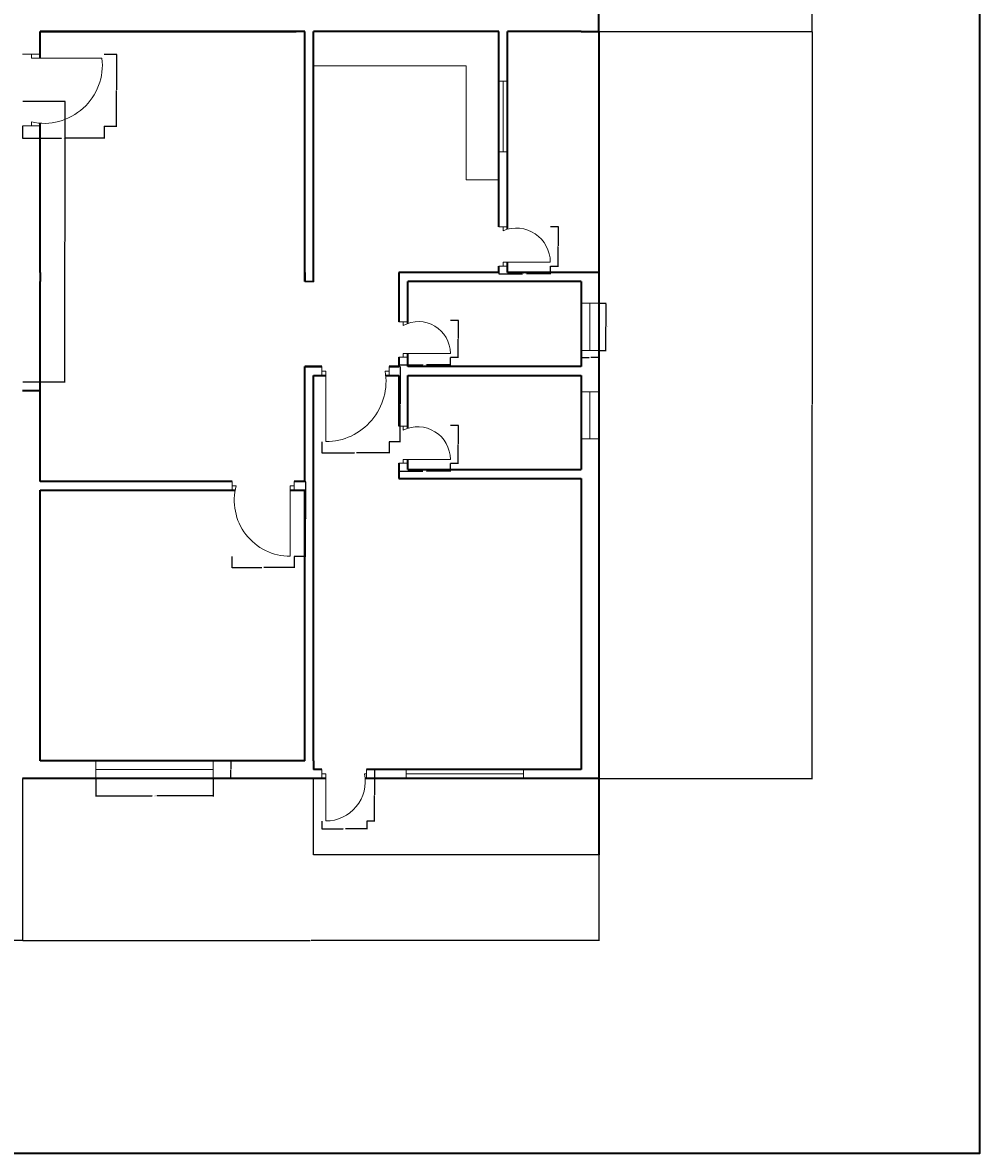
# Model space of a CAD drawing. Units: inches. Extents: x 2120 to 4013, y 1390 to 3019.
# Tile 51 of 59: x 3525 to 4013, y 1390 to 1967. Entities that reach past the tile are written whole.
import ezdxf

# ---------------------------------------------------------------- set-up
doc = ezdxf.new("R2010")
doc.units = ezdxf.units.IN
for name, color, linetype, lineweight in [('A-ANNO-DIMS', 2, 'Continuous', 18), ('A-ANNO-TTLB', 7, 'Continuous', 35), ('A-DOOR', 3, 'Continuous', 18), ('A-FLOR-CASE', 8, 'Continuous', 18), ('A-FLOR-DECK', 7, 'Continuous', 25), ('A-FURN', 8, 'Continuous', 13), ('A-GLAZ', 4, 'Continuous', 18), ('A-WALL', 7, 'Continuous', 35)]:
    doc.layers.add(name, color=color, linetype=linetype, lineweight=lineweight)
doc.styles.get("Standard").update_dxf_attribs({"font": 'arial.ttf'})
doc.dimstyles.get("Standard").update_dxf_attribs({"dimtxt": 0.18, "dimasz": 0.18, "dimexe": 0.18, "dimexo": 0.0625, "dimgap": 0.09, "dimtad": 0, "dimtih": 1, "dimtoh": 1, "dimdec": 4, "dimzin": 0, "dimdsep": 46, "dimtxsty": 'Standard', "dimcen": 0.09, "dimadec": 0, "dimazin": 0, "dimtfac": 1, "dimtdec": 4, "dimtofl": 0, "dimtmove": 0, "dimatfit": 3, "dimfxl": 1, "dimtolj": 1, "dimtzin": 0, "dimarcsym": 0})

# ---------------------------------------------------------------- blocks, each defined once
blk = doc.blocks.new('DOOR-SWING-24IN-116p21DEG')
for p, q in [((0, 18.94), (4.5, 18.94)), ((4.5, 18.94), (2.25, 18.94)), ((2.25, 18.94), (2.25, 16.94)), ((4.5, 0), (0, 0)), ((0, 0), (2.25, 0)), ((2.25, 0), (2.25, 2)), ((2.25, 2), (26.25, 2))]:
    blk.add_line(p, q)
blk.add_arc((9.6, 2), 16.65, 0, 116.20868)
blk = doc.blocks.new('DOOR-SWING-24IN-119p01DEG')
for p, q in [((0, 18.13), (4.5, 18.13)), ((4.5, 18.13), (2.25, 18.13)), ((2.25, 18.13), (2.25, 16.13)), ((0, 0), (4.5, 0)), ((2.25, 0), (2.25, 2)), ((2.25, 2), (26.25, 2)), ((4.5, 0), (2.25, 0))]:
    blk.add_line(p, q)
blk.add_arc((10.09, 2), 16.16, 0, 119.01366)
blk = doc.blocks.new('DOOR-SWING-24IN-100p95DEG')
for p, q in [((0, 26.25), (0, 21.75)), ((0, 21.75), (0, 24)), ((0, 24), (2, 24)), ((2, 24), (2, 0)), ((22.8, 24), (21.8, 24)), ((22.8, 26.25), (22.8, 21.75)), ((22.8, 21.75), (22.8, 24))]:
    blk.add_line(p, q)
blk.add_arc((2, 20.17), 20.17, 270, 10.95076)
blk = doc.blocks.new('DOOR-SWING-24IN-112p55DEG')
for p, q in [((0, 20.02), (4.5, 20.02)), ((4.5, 20.02), (2.25, 20.02)), ((2.25, 20.02), (2.25, 18.02)), ((0, 0), (4.5, 0)), ((2.25, 0), (2.25, 2)), ((2.25, 2), (26.25, 2)), ((4.5, 0), (2.25, 0))]:
    blk.add_line(p, q)
blk.add_arc((8.9, 2), 17.35, 0, 112.55014)
blk = doc.blocks.new('DOOR-SWING-36IN-99p84DEG')
for p, q in [((0, 38.25), (0, 33.75)), ((0, 33.75), (0, 38.25)), ((0, 38.25), (0, 36)), ((0, 36), (2, 36)), ((2, 36), (2, 0)), ((34.3, 36), (32.3, 36)), ((34.3, 38.25), (34.3, 33.75)), ((34.3, 33.75), (34.3, 36))]:
    blk.add_line(p, q)
blk.add_arc((2, 30.75), 30.75, 270, 9.83553)
blk = doc.blocks.new('DOOR-SWING-36IN-105p06DEG')
for p, q in [((0, 33.75), (0, 38.25)), ((0, 38.25), (0, 36)), ((0, 36), (2, 36)), ((31.6, 36), (29.6, 36)), ((29.6, 36), (29.6, 0)), ((31.6, 38.25), (31.6, 33.75)), ((31.6, 33.75), (31.6, 36))]:
    blk.add_line(p, q)
blk.add_arc((29.6, 28.58), 28.58, 164.94449, 270)
blk = doc.blocks.new('DOOR-SWING-36IN-109p07DEG')
for p, q in [((9, 36.56), (0, 36.56)), ((0, 36.56), (4.5, 36.56)), ((4.5, 36.56), (4.5, 34.56)), ((9, 36.56), (9, 36.56)), ((4.5, 34.56), (40.5, 34.56)), ((9, 0), (0, 0)), ((0, 0), (4.5, 0)), ((4.5, 0), (4.5, 2))]:
    blk.add_line(p, q)
blk.add_arc((10.9, 31.1), 29.8, 257.59275, 6.66524)
blk = doc.blocks.new('WIN-PLAN-24IN-03')
for p, q in [((9, 24), (0, 24)), ((0, 24), (4.5, 24)), ((4.5, 24), (4.5, 0)), ((9, 0), (0, 0)), ((4.5, 0), (9, 0))]:
    blk.add_line(p, q)
blk = doc.blocks.new('WIN-PLAN-24IN-05')
for p, q in [((4.5, 24), (0, 24)), ((0, 24), (9, 24)), ((4.5, 0), (4.5, 24)), ((0, 0), (9, 0)), ((9, 0), (0, 0)), ((0, 0), (4.5, 0))]:
    blk.add_line(p, q)
blk = doc.blocks.new('WIN-PLAN-60IN-03')
for p, q in [((0, 4.5), (0, 0)), ((0, 0), (0, 2.25)), ((0, 2.25), (60, 2.25)), ((60, 2.25), (60, 4.5)), ((60, 4.5), (60, 0))]:
    blk.add_line(p, q)
blk = doc.blocks.new('WIN-PLAN-60IN-04')
for p, q in [((0, 9), (0, 9)), ((0, 9), (0, 0)), ((60, 4.5), (60, 9)), ((60, 9), (60, 0)), ((0, 0), (0, 4.5)), ((0, 4.5), (60, 4.5))]:
    blk.add_line(p, q)
blk = doc.blocks.new('WIN-PLAN-36IN-02')
for p, q in [((2.25, 36), (0, 36)), ((0, 36), (4.5, 36)), ((2.25, 0), (2.25, 36)), ((0, 0), (4.5, 0)), ((4.5, 0), (2.25, 0))]:
    blk.add_line(p, q)
blk = doc.blocks.new('*D79')
at = {"layer": 'A-ANNO-DIMS', "color": 0, "lineweight": -2, "transparency": 16777216}
for p, q in [((3524.8, 1926.95), (3546.38, 1926.95)), ((3546.2, 1926.77), (3546.2, 1855.58)), ((3546.2, 1784.02), (3546.2, 1855.21)), ((3524.8, 1783.84), (3546.38, 1783.84))]:
    blk.add_line(p, q, dxfattribs=at)
at = {"layer": 'A-ANNO-DIMS', "color": 0, "transparency": 16777216}
for points in [[(3546.17, 1926.77), (3546.23, 1926.77), (3546.2, 1926.95)], [(3546.17, 1784.02), (3546.23, 1784.02), (3546.2, 1783.84)]]:
    blk.add_solid(points, dxfattribs=at)
at = {"layer": 'Defpoints', "color": 0, "transparency": 16777216}
for p in [(3524.73, 1926.95), (3546.2, 1926.95), (3524.73, 1783.84)]:
    blk.add_point(p, dxfattribs=at)
at = {"layer": 'A-ANNO-DIMS', "color": 0, "transparency": 16777216, "insert": (3546.2, 1855.39), "char_height": 0.18, "attachment_point": 5}
blk.add_mtext('\\A1;STAIR 143 TYP.', dxfattribs=at)
blk = doc.blocks.new('*D127')
at = {"layer": 'A-ANNO-DIMS', "color": 0, "lineweight": -2, "transparency": 16777216}
for p, q in [((3716.73, 1742.16), (3716.73, 1738.11)), ((3742.98, 1742.16), (3742.98, 1738.11)), ((3716.91, 1738.29), (3728.87, 1738.29)), ((3742.8, 1738.29), (3730.85, 1738.29))]:
    blk.add_line(p, q, dxfattribs=at)
at = {"layer": 'A-ANNO-DIMS', "color": 0, "transparency": 16777216}
for points in [[(3716.91, 1738.32), (3716.91, 1738.26), (3716.73, 1738.29)], [(3742.8, 1738.32), (3742.8, 1738.26), (3742.98, 1738.29)]]:
    blk.add_solid(points, dxfattribs=at)
at = {"layer": 'Defpoints', "color": 0, "transparency": 16777216}
for p in [(3716.73, 1742.23), (3742.98, 1742.23), (3742.98, 1738.29)]:
    blk.add_point(p, dxfattribs=at)
at = {"layer": 'A-ANNO-DIMS', "color": 0, "transparency": 16777216, "insert": (3729.86, 1738.29), "char_height": 0.18, "attachment_point": 5}
blk.add_mtext('\\A1;SWING 26 TYP.', dxfattribs=at)
blk = doc.blocks.new('*D128')
at = {"layer": 'A-ANNO-DIMS', "color": 0, "lineweight": -2, "transparency": 16777216}
for p, q in [((3743.05, 1761.7), (3747.1, 1761.7)), ((3746.92, 1761.52), (3746.92, 1752.15)), ((3746.92, 1742.41), (3746.92, 1751.78)), ((3743.05, 1742.23), (3747.1, 1742.23))]:
    blk.add_line(p, q, dxfattribs=at)
at = {"layer": 'A-ANNO-DIMS', "color": 0, "transparency": 16777216}
for points in [[(3746.89, 1761.52), (3746.95, 1761.52), (3746.92, 1761.7)], [(3746.89, 1742.41), (3746.95, 1742.41), (3746.92, 1742.23)]]:
    blk.add_solid(points, dxfattribs=at)
at = {"layer": 'Defpoints', "color": 0, "transparency": 16777216}
for p in [(3742.98, 1761.7), (3746.92, 1761.7), (3742.98, 1742.23)]:
    blk.add_point(p, dxfattribs=at)
at = {"layer": 'A-ANNO-DIMS', "color": 0, "transparency": 16777216, "insert": (3746.92, 1751.96), "char_height": 0.18, "attachment_point": 5}
blk.add_mtext('\\A1;19 TYP.', dxfattribs=at)
blk = doc.blocks.new('*D129')
at = {"layer": 'A-ANNO-DIMS', "color": 0, "lineweight": -2, "transparency": 16777216}
for p, q in [((3716.73, 1796.26), (3716.73, 1792.21)), ((3742.98, 1796.26), (3742.98, 1792.21)), ((3716.91, 1792.39), (3728.87, 1792.39)), ((3742.8, 1792.39), (3730.85, 1792.39))]:
    blk.add_line(p, q, dxfattribs=at)
at = {"layer": 'A-ANNO-DIMS', "color": 0, "transparency": 16777216}
for points in [[(3716.91, 1792.42), (3716.91, 1792.36), (3716.73, 1792.39)], [(3742.8, 1792.42), (3742.8, 1792.36), (3742.98, 1792.39)]]:
    blk.add_solid(points, dxfattribs=at)
at = {"layer": 'Defpoints', "color": 0, "transparency": 16777216}
for p in [(3716.73, 1796.33), (3742.98, 1796.33), (3742.98, 1792.39)]:
    blk.add_point(p, dxfattribs=at)
at = {"layer": 'A-ANNO-DIMS', "color": 0, "transparency": 16777216, "insert": (3729.86, 1792.39), "char_height": 0.18, "attachment_point": 5}
blk.add_mtext('\\A1;SWING 26 TYP.', dxfattribs=at)
blk = doc.blocks.new('*D130')
at = {"layer": 'A-ANNO-DIMS', "color": 0, "lineweight": -2, "transparency": 16777216}
for p, q in [((3743.05, 1815.24), (3747.1, 1815.24)), ((3746.92, 1815.06), (3746.92, 1805.96)), ((3746.92, 1796.51), (3746.92, 1805.6)), ((3743.05, 1796.33), (3747.1, 1796.33))]:
    blk.add_line(p, q, dxfattribs=at)
at = {"layer": 'A-ANNO-DIMS', "color": 0, "transparency": 16777216}
for points in [[(3746.89, 1815.06), (3746.95, 1815.06), (3746.92, 1815.24)], [(3746.89, 1796.51), (3746.95, 1796.51), (3746.92, 1796.33)]]:
    blk.add_solid(points, dxfattribs=at)
at = {"layer": 'Defpoints', "color": 0, "transparency": 16777216}
for p in [(3742.98, 1815.24), (3746.92, 1815.24), (3742.98, 1796.33)]:
    blk.add_point(p, dxfattribs=at)
at = {"layer": 'A-ANNO-DIMS', "color": 0, "transparency": 16777216, "insert": (3746.92, 1805.78), "char_height": 0.18, "attachment_point": 5}
blk.add_mtext('\\A1;19 TYP.', dxfattribs=at)
blk = doc.blocks.new('*D131')
at = {"layer": 'A-ANNO-DIMS', "color": 0, "lineweight": -2, "transparency": 16777216}
for p, q in [((3700.42, 1586.03), (3704.48, 1586.03)), ((3704.3, 1585.85), (3704.3, 1573.09)), ((3704.3, 1559.96), (3704.3, 1572.72)), ((3700.42, 1559.78), (3704.48, 1559.78))]:
    blk.add_line(p, q, dxfattribs=at)
at = {"layer": 'A-ANNO-DIMS', "color": 0, "transparency": 16777216}
for points in [[(3704.27, 1585.85), (3704.33, 1585.85), (3704.3, 1586.03)], [(3704.27, 1559.96), (3704.33, 1559.96), (3704.3, 1559.78)]]:
    blk.add_solid(points, dxfattribs=at)
at = {"layer": 'Defpoints', "color": 0, "transparency": 16777216}
for p in [(3700.36, 1586.03), (3704.3, 1586.03), (3700.36, 1559.78)]:
    blk.add_point(p, dxfattribs=at)
at = {"layer": 'A-ANNO-DIMS', "color": 0, "transparency": 16777216, "insert": (3704.3, 1572.91), "char_height": 0.18, "attachment_point": 5}
blk.add_mtext('\\A1;SWING 26 TYP.', dxfattribs=at)
blk = doc.blocks.new('*D132')
at = {"layer": 'A-ANNO-DIMS', "color": 0, "lineweight": -2, "transparency": 16777216}
for p, q in [((3677.41, 1559.72), (3677.41, 1555.66)), ((3700.36, 1559.72), (3700.36, 1555.66)), ((3677.59, 1555.84), (3688.36, 1555.84)), ((3700.18, 1555.84), (3689.42, 1555.84))]:
    blk.add_line(p, q, dxfattribs=at)
at = {"layer": 'A-ANNO-DIMS', "color": 0, "transparency": 16777216}
for points in [[(3677.59, 1555.87), (3677.59, 1555.81), (3677.41, 1555.84)], [(3700.18, 1555.87), (3700.18, 1555.81), (3700.36, 1555.84)]]:
    blk.add_solid(points, dxfattribs=at)
at = {"layer": 'Defpoints', "color": 0, "transparency": 16777216}
for p in [(3677.41, 1559.78), (3700.36, 1559.78), (3700.36, 1555.84)]:
    blk.add_point(p, dxfattribs=at)
at = {"layer": 'A-ANNO-DIMS', "color": 0, "transparency": 16777216, "insert": (3688.89, 1555.84), "char_height": 0.18, "attachment_point": 5}
blk.add_mtext('\\A1;23 TYP.', dxfattribs=at)
blk = doc.blocks.new('*D133')
at = {"layer": 'A-ANNO-DIMS', "color": 0, "lineweight": -2, "transparency": 16777216}
for p, q in [((3767.73, 1842.8), (3767.73, 1838.75)), ((3793.98, 1842.8), (3793.98, 1838.75)), ((3767.91, 1838.93), (3779.87, 1838.93)), ((3793.8, 1838.93), (3781.85, 1838.93))]:
    blk.add_line(p, q, dxfattribs=at)
at = {"layer": 'A-ANNO-DIMS', "color": 0, "transparency": 16777216}
for points in [[(3767.91, 1838.96), (3767.91, 1838.9), (3767.73, 1838.93)], [(3793.8, 1838.96), (3793.8, 1838.9), (3793.98, 1838.93)]]:
    blk.add_solid(points, dxfattribs=at)
at = {"layer": 'Defpoints', "color": 0, "transparency": 16777216}
for p in [(3767.73, 1842.86), (3793.98, 1842.86), (3793.98, 1838.93)]:
    blk.add_point(p, dxfattribs=at)
at = {"layer": 'A-ANNO-DIMS', "color": 0, "transparency": 16777216, "insert": (3780.86, 1838.93), "char_height": 0.18, "attachment_point": 5}
blk.add_mtext('\\A1;SWING 26 TYP.', dxfattribs=at)
blk = doc.blocks.new('*D134')
at = {"layer": 'A-ANNO-DIMS', "color": 0, "lineweight": -2, "transparency": 16777216}
for p, q in [((3794.05, 1863.11), (3798.1, 1863.11)), ((3797.92, 1862.93), (3797.92, 1853.17)), ((3797.92, 1843.04), (3797.92, 1852.8)), ((3794.05, 1842.86), (3798.1, 1842.86))]:
    blk.add_line(p, q, dxfattribs=at)
at = {"layer": 'A-ANNO-DIMS', "color": 0, "transparency": 16777216}
for points in [[(3797.89, 1862.93), (3797.95, 1862.93), (3797.92, 1863.11)], [(3797.89, 1843.04), (3797.95, 1843.04), (3797.92, 1842.86)]]:
    blk.add_solid(points, dxfattribs=at)
at = {"layer": 'Defpoints', "color": 0, "transparency": 16777216}
for p in [(3793.98, 1863.11), (3797.92, 1863.11), (3793.98, 1842.86)]:
    blk.add_point(p, dxfattribs=at)
at = {"layer": 'A-ANNO-DIMS', "color": 0, "transparency": 16777216, "insert": (3797.92, 1852.99), "char_height": 0.18, "attachment_point": 5}
blk.add_mtext('\\A1;20 TYP.', dxfattribs=at)
blk = doc.blocks.new('*D157')
at = {"layer": 'A-ANNO-DIMS', "color": 0, "lineweight": -2, "transparency": 16777216}
for p, q in [((3711.77, 1791.53), (3717.62, 1791.53)), ((3717.44, 1791.35), (3717.44, 1772.59)), ((3717.44, 1753.46), (3717.44, 1772.22)), ((3711.77, 1753.28), (3717.62, 1753.28))]:
    blk.add_line(p, q, dxfattribs=at)
at = {"layer": 'A-ANNO-DIMS', "color": 0, "transparency": 16777216}
for points in [[(3717.41, 1791.35), (3717.47, 1791.35), (3717.44, 1791.53)], [(3717.41, 1753.46), (3717.47, 1753.46), (3717.44, 1753.28)]]:
    blk.add_solid(points, dxfattribs=at)
at = {"layer": 'Defpoints', "color": 0, "transparency": 16777216}
for p in [(3711.7, 1791.53), (3717.44, 1791.53), (3711.7, 1753.28)]:
    blk.add_point(p, dxfattribs=at)
at = {"layer": 'A-ANNO-DIMS', "color": 0, "transparency": 16777216, "insert": (3717.44, 1772.41), "char_height": 0.18, "attachment_point": 5}
blk.add_mtext('\\A1;SWING 38 TYP.', dxfattribs=at)
blk = doc.blocks.new('*D158')
at = {"layer": 'A-ANNO-DIMS', "color": 0, "lineweight": -2, "transparency": 16777216}
for p, q in [((3677.41, 1753.22), (3677.41, 1747.36)), ((3711.7, 1753.22), (3711.7, 1747.36)), ((3677.59, 1747.54), (3694.03, 1747.54)), ((3711.52, 1747.54), (3695.08, 1747.54))]:
    blk.add_line(p, q, dxfattribs=at)
at = {"layer": 'A-ANNO-DIMS', "color": 0, "transparency": 16777216}
for points in [[(3677.59, 1747.57), (3677.59, 1747.51), (3677.41, 1747.54)], [(3711.52, 1747.57), (3711.52, 1747.51), (3711.7, 1747.54)]]:
    blk.add_solid(points, dxfattribs=at)
at = {"layer": 'Defpoints', "color": 0, "transparency": 16777216}
for p in [(3677.41, 1753.28), (3711.7, 1753.28), (3711.7, 1747.54)]:
    blk.add_point(p, dxfattribs=at)
at = {"layer": 'A-ANNO-DIMS', "color": 0, "transparency": 16777216, "insert": (3694.56, 1747.54), "char_height": 0.18, "attachment_point": 5}
blk.add_mtext('\\A1;34 TYP.', dxfattribs=at)
blk = doc.blocks.new('*D159')
at = {"layer": 'A-ANNO-DIMS', "color": 0, "lineweight": -2, "transparency": 16777216}
for p, q in [((3663.38, 1733.03), (3669.23, 1733.03)), ((3669.05, 1732.85), (3669.05, 1714.09)), ((3669.05, 1694.96), (3669.05, 1713.72)), ((3663.38, 1694.78), (3669.23, 1694.78))]:
    blk.add_line(p, q, dxfattribs=at)
at = {"layer": 'A-ANNO-DIMS', "color": 0, "transparency": 16777216}
for points in [[(3669.02, 1732.85), (3669.08, 1732.85), (3669.05, 1733.03)], [(3669.02, 1694.96), (3669.08, 1694.96), (3669.05, 1694.78)]]:
    blk.add_solid(points, dxfattribs=at)
at = {"layer": 'Defpoints', "color": 0, "transparency": 16777216}
for p in [(3663.31, 1733.03), (3669.05, 1733.03), (3663.31, 1694.78)]:
    blk.add_point(p, dxfattribs=at)
at = {"layer": 'A-ANNO-DIMS', "color": 0, "transparency": 16777216, "insert": (3669.05, 1713.91), "char_height": 0.18, "attachment_point": 5}
blk.add_mtext('\\A1;SWING 38 TYP.', dxfattribs=at)
blk = doc.blocks.new('*D160')
at = {"layer": 'A-ANNO-DIMS', "color": 0, "lineweight": -2, "transparency": 16777216}
for p, q in [((3631.41, 1694.72), (3631.41, 1688.86)), ((3663.31, 1694.72), (3663.31, 1688.86)), ((3631.59, 1689.04), (3646.83, 1689.04)), ((3663.13, 1689.04), (3647.89, 1689.04))]:
    blk.add_line(p, q, dxfattribs=at)
at = {"layer": 'A-ANNO-DIMS', "color": 0, "transparency": 16777216}
for points in [[(3631.59, 1689.07), (3631.59, 1689.01), (3631.41, 1689.04)], [(3663.13, 1689.07), (3663.13, 1689.01), (3663.31, 1689.04)]]:
    blk.add_solid(points, dxfattribs=at)
at = {"layer": 'Defpoints', "color": 0, "transparency": 16777216}
for p in [(3631.41, 1694.78), (3663.31, 1694.78), (3663.31, 1689.04)]:
    blk.add_point(p, dxfattribs=at)
at = {"layer": 'A-ANNO-DIMS', "color": 0, "transparency": 16777216, "insert": (3647.36, 1689.04), "char_height": 0.18, "attachment_point": 5}
blk.add_mtext('\\A1;32 TYP.', dxfattribs=at)
blk = doc.blocks.new('*D161')
at = {"layer": 'A-ANNO-DIMS', "color": 0, "lineweight": -2, "transparency": 16777216}
for p, q in [((3524.73, 1914.21), (3524.73, 1907.85)), ((3566.35, 1914.21), (3566.35, 1907.85)), ((3524.91, 1908.03), (3544.56, 1908.03)), ((3566.17, 1908.03), (3546.53, 1908.03))]:
    blk.add_line(p, q, dxfattribs=at)
at = {"layer": 'A-ANNO-DIMS', "color": 0, "transparency": 16777216}
for points in [[(3524.91, 1908.06), (3524.91, 1908), (3524.73, 1908.03)], [(3566.17, 1908.06), (3566.17, 1908), (3566.35, 1908.03)]]:
    blk.add_solid(points, dxfattribs=at)
at = {"layer": 'Defpoints', "color": 0, "transparency": 16777216}
for p in [(3524.73, 1914.27), (3566.35, 1914.27), (3566.35, 1908.03)]:
    blk.add_point(p, dxfattribs=at)
at = {"layer": 'A-ANNO-DIMS', "color": 0, "transparency": 16777216, "insert": (3545.54, 1908.03), "char_height": 0.18, "attachment_point": 5}
blk.add_mtext('\\A1;SWING 42 TYP.', dxfattribs=at)
blk = doc.blocks.new('*D162')
at = {"layer": 'A-ANNO-DIMS', "color": 0, "lineweight": -2, "transparency": 16777216}
for p, q in [((3566.42, 1950.9), (3572.78, 1950.9)), ((3572.6, 1950.72), (3572.6, 1932.77)), ((3572.6, 1914.45), (3572.6, 1932.41)), ((3566.42, 1914.27), (3572.78, 1914.27))]:
    blk.add_line(p, q, dxfattribs=at)
at = {"layer": 'A-ANNO-DIMS', "color": 0, "transparency": 16777216}
for points in [[(3572.57, 1950.72), (3572.63, 1950.72), (3572.6, 1950.9)], [(3572.57, 1914.45), (3572.63, 1914.45), (3572.6, 1914.27)]]:
    blk.add_solid(points, dxfattribs=at)
at = {"layer": 'Defpoints', "color": 0, "transparency": 16777216}
for p in [(3566.35, 1950.9), (3572.6, 1950.9), (3566.35, 1914.27)]:
    blk.add_point(p, dxfattribs=at)
at = {"layer": 'A-ANNO-DIMS', "color": 0, "transparency": 16777216, "insert": (3572.6, 1932.59), "char_height": 0.18, "attachment_point": 5}
blk.add_mtext('\\A1;37 TYP.', dxfattribs=at)
blk = doc.blocks.new('*D185')
at = {"layer": 'A-ANNO-DIMS', "color": 0, "lineweight": -2, "transparency": 16777216}
for p, q in [((3818.8, 1823.84), (3822.51, 1823.84)), ((3822.33, 1823.66), (3822.33, 1812.03)), ((3822.33, 1800.02), (3822.33, 1811.66)), ((3818.8, 1799.84), (3822.51, 1799.84))]:
    blk.add_line(p, q, dxfattribs=at)
at = {"layer": 'A-ANNO-DIMS', "color": 0, "transparency": 16777216}
for points in [[(3822.3, 1823.66), (3822.36, 1823.66), (3822.33, 1823.84)], [(3822.3, 1800.02), (3822.36, 1800.02), (3822.33, 1799.84)]]:
    blk.add_solid(points, dxfattribs=at)
at = {"layer": 'Defpoints', "color": 0, "transparency": 16777216}
for p in [(3818.73, 1823.84), (3822.33, 1823.84), (3818.73, 1799.84)]:
    blk.add_point(p, dxfattribs=at)
at = {"layer": 'A-ANNO-DIMS', "color": 0, "transparency": 16777216, "insert": (3822.33, 1811.84), "char_height": 0.18, "attachment_point": 5}
blk.add_mtext('\\A1;WINDOW 24 TYP.', dxfattribs=at)
blk = doc.blocks.new('*D186')
at = {"layer": 'A-ANNO-DIMS', "color": 0, "lineweight": -2, "transparency": 16777216}
for p, q in [((3809.73, 1799.78), (3809.73, 1796.06)), ((3818.73, 1799.78), (3818.73, 1796.06)), ((3809.91, 1796.24), (3813.78, 1796.24)), ((3818.55, 1796.24), (3814.69, 1796.24))]:
    blk.add_line(p, q, dxfattribs=at)
at = {"layer": 'A-ANNO-DIMS', "color": 0, "transparency": 16777216}
for points in [[(3809.91, 1796.27), (3809.91, 1796.21), (3809.73, 1796.24)], [(3818.55, 1796.27), (3818.55, 1796.21), (3818.73, 1796.24)]]:
    blk.add_solid(points, dxfattribs=at)
at = {"layer": 'Defpoints', "color": 0, "transparency": 16777216}
for p in [(3809.73, 1799.84), (3818.73, 1799.84), (3818.73, 1796.24)]:
    blk.add_point(p, dxfattribs=at)
at = {"layer": 'A-ANNO-DIMS', "color": 0, "transparency": 16777216, "insert": (3814.23, 1796.24), "char_height": 0.18, "attachment_point": 5}
blk.add_mtext('\\A1;9 TYP.', dxfattribs=at)
blk = doc.blocks.new('*D189')
at = {"layer": 'A-ANNO-DIMS', "color": 0, "lineweight": -2, "transparency": 16777216}
for p, q in [((3562.02, 1581.47), (3562.02, 1572.35)), ((3622.02, 1581.47), (3622.02, 1572.35)), ((3562.2, 1572.53), (3590.9, 1572.53)), ((3621.84, 1572.53), (3593.14, 1572.53))]:
    blk.add_line(p, q, dxfattribs=at)
at = {"layer": 'A-ANNO-DIMS', "color": 0, "transparency": 16777216}
for points in [[(3562.2, 1572.56), (3562.2, 1572.5), (3562.02, 1572.53)], [(3621.84, 1572.56), (3621.84, 1572.5), (3622.02, 1572.53)]]:
    blk.add_solid(points, dxfattribs=at)
at = {"layer": 'Defpoints', "color": 0, "transparency": 16777216}
for p in [(3562.02, 1581.53), (3622.02, 1581.53), (3622.02, 1572.53)]:
    blk.add_point(p, dxfattribs=at)
at = {"layer": 'A-ANNO-DIMS', "color": 0, "transparency": 16777216, "insert": (3592.02, 1572.53), "char_height": 0.18, "attachment_point": 5}
blk.add_mtext('\\A1;WINDOW 60 TYP.', dxfattribs=at)
blk = doc.blocks.new('*D190')
at = {"layer": 'A-ANNO-DIMS', "color": 0, "lineweight": -2, "transparency": 16777216}
for p, q in [((3622.08, 1590.53), (3631.2, 1590.53)), ((3631.02, 1590.35), (3631.02, 1586.21)), ((3622.08, 1581.53), (3631.2, 1581.53)), ((3631.02, 1581.71), (3631.02, 1585.85))]:
    blk.add_line(p, q, dxfattribs=at)
at = {"layer": 'A-ANNO-DIMS', "color": 0, "transparency": 16777216}
for points in [[(3630.99, 1590.35), (3631.05, 1590.35), (3631.02, 1590.53)], [(3630.99, 1581.71), (3631.05, 1581.71), (3631.02, 1581.53)]]:
    blk.add_solid(points, dxfattribs=at)
at = {"layer": 'Defpoints', "color": 0, "transparency": 16777216}
for p in [(3622.02, 1590.53), (3631.02, 1590.53), (3622.02, 1581.53)]:
    blk.add_point(p, dxfattribs=at)
at = {"layer": 'A-ANNO-DIMS', "color": 0, "transparency": 16777216, "insert": (3631.02, 1586.03), "char_height": 0.18, "attachment_point": 5}
blk.add_mtext('\\A1;9 TYP.', dxfattribs=at)
blk = doc.blocks.new('*D218')
at = {"layer": 'A-ANNO-DIMS', "color": 0, "lineweight": -2, "transparency": 16777216}
for p, q in [((3818.8, 2352.53), (3927.73, 2352.53)), ((3927.55, 2352.35), (3927.55, 2157.71)), ((3927.55, 1962.71), (3927.55, 2157.35)), ((3818.8, 1962.53), (3927.73, 1962.53))]:
    blk.add_line(p, q, dxfattribs=at)
at = {"layer": 'A-ANNO-DIMS', "color": 0, "transparency": 16777216}
for points in [[(3927.52, 2352.35), (3927.58, 2352.35), (3927.55, 2352.53)], [(3927.52, 1962.71), (3927.58, 1962.71), (3927.55, 1962.53)]]:
    blk.add_solid(points, dxfattribs=at)
at = {"layer": 'Defpoints', "color": 0, "transparency": 16777216}
for p in [(3818.73, 2352.53), (3818.73, 1962.53), (3927.55, 1962.53)]:
    blk.add_point(p, dxfattribs=at)
at = {"layer": 'A-ANNO-DIMS', "color": 0, "transparency": 16777216, "insert": (3927.55, 2157.53), "char_height": 0.18, "attachment_point": 5}
blk.add_mtext('\\A1;390', dxfattribs=at)
blk = doc.blocks.new('*D219')
at = {"layer": 'A-ANNO-DIMS', "color": 0, "lineweight": -2, "transparency": 16777216}
for p, q in [((3818.8, 1962.53), (3927.73, 1962.53)), ((3927.55, 1962.35), (3927.55, 1772.21)), ((3927.55, 1581.71), (3927.55, 1771.85)), ((3818.8, 1581.53), (3927.73, 1581.53))]:
    blk.add_line(p, q, dxfattribs=at)
at = {"layer": 'A-ANNO-DIMS', "color": 0, "transparency": 16777216}
for points in [[(3927.52, 1962.35), (3927.58, 1962.35), (3927.55, 1962.53)], [(3927.52, 1581.71), (3927.58, 1581.71), (3927.55, 1581.53)]]:
    blk.add_solid(points, dxfattribs=at)
at = {"layer": 'Defpoints', "color": 0, "transparency": 16777216}
for p in [(3818.73, 1962.53), (3818.73, 1581.53), (3927.55, 1581.53)]:
    blk.add_point(p, dxfattribs=at)
at = {"layer": 'A-ANNO-DIMS', "color": 0, "transparency": 16777216, "insert": (3927.55, 1772.03), "char_height": 0.18, "attachment_point": 5}
blk.add_mtext('\\A1;381', dxfattribs=at)
blk = doc.blocks.new('*D221')
at = {"layer": 'A-ANNO-DIMS', "color": 0, "lineweight": -2, "transparency": 16777216}
for p, q in [((3524.73, 1581.47), (3524.73, 1498.6)), ((3446.73, 1542.47), (3446.73, 1498.6)), ((3446.91, 1498.78), (3485.52, 1498.78)), ((3524.55, 1498.78), (3485.95, 1498.78))]:
    blk.add_line(p, q, dxfattribs=at)
at = {"layer": 'A-ANNO-DIMS', "color": 0, "transparency": 16777216}
for points in [[(3446.91, 1498.81), (3446.91, 1498.75), (3446.73, 1498.78)], [(3524.55, 1498.81), (3524.55, 1498.75), (3524.73, 1498.78)]]:
    blk.add_solid(points, dxfattribs=at)
at = {"layer": 'Defpoints', "color": 0, "transparency": 16777216}
for p in [(3524.73, 1581.53), (3446.73, 1542.53), (3524.73, 1498.78)]:
    blk.add_point(p, dxfattribs=at)
at = {"layer": 'A-ANNO-DIMS', "color": 0, "transparency": 16777216, "insert": (3485.73, 1498.78), "char_height": 0.18, "attachment_point": 5}
blk.add_mtext('\\A1;78', dxfattribs=at)
blk = doc.blocks.new('*D222')
at = {"layer": 'A-ANNO-DIMS', "color": 0, "lineweight": -2, "transparency": 16777216}
for p, q in [((3524.73, 1581.47), (3524.73, 1498.6)), ((3818.73, 1542.47), (3818.73, 1498.6)), ((3524.91, 1498.78), (3671.44, 1498.78)), ((3818.55, 1498.78), (3672.02, 1498.78))]:
    blk.add_line(p, q, dxfattribs=at)
at = {"layer": 'A-ANNO-DIMS', "color": 0, "transparency": 16777216}
for points in [[(3524.91, 1498.81), (3524.91, 1498.75), (3524.73, 1498.78)], [(3818.55, 1498.81), (3818.55, 1498.75), (3818.73, 1498.78)]]:
    blk.add_solid(points, dxfattribs=at)
at = {"layer": 'Defpoints', "color": 0, "transparency": 16777216}
for p in [(3524.73, 1581.53), (3818.73, 1542.53), (3818.73, 1498.78)]:
    blk.add_point(p, dxfattribs=at)
at = {"layer": 'A-ANNO-DIMS', "color": 0, "transparency": 16777216, "insert": (3671.73, 1498.78), "char_height": 0.18, "attachment_point": 5}
blk.add_mtext('\\A1;294', dxfattribs=at)

msp = doc.modelspace()

# ---------------------------------------------------------------- linework, layer by layer
at = {"layer": 'A-ANNO-TTLB'}
msp.add_lwpolyline([(2120.4581, 3019.1237), (4012.9334, 3019.1237), (4012.9334, 1390.2222), (2120.4581, 1390.2222)], close=True, dxfattribs=at)
at = {"layer": 'A-FLOR-CASE'}
for p, q in [((3673.2347, 1944.9893), (3751.0537, 1944.9893)), ((3751.0537, 1944.9893), (3751.0537, 1886.7683)), ((3751.0537, 1886.7683), (3767.7347, 1886.7683))]:
    msp.add_line(p, q, dxfattribs=at)
at = {"layer": 'A-FLOR-DECK'}
for p, q in [((3673.2347, 1542.531), (3673.2347, 1581.531)), ((3818.7347, 1542.531), (3673.2347, 1542.531))]:
    msp.add_line(p, q, dxfattribs=at)
at = {"layer": 'A-FURN'}
for p, q in [((3809.7347, 1684.8087), (3809.7347, 1637.0184)), ((3533.7347, 1633.5966), (3533.7347, 1681.3869))]:
    msp.add_line(p, q, dxfattribs=at)
at = {"layer": 'A-WALL'}
for p, q in [((3818.7347, 1962.531), (3818.7347, 1971.531)), ((3668.7347, 1962.531), (3533.7347, 1962.531)), ((3533.7347, 1948.9035), (3533.7347, 1962.531)), ((3533.7347, 1962.531), (3664.2347, 1962.531)), ((3668.7347, 1835.031), (3668.7347, 1962.531)), ((3673.2347, 1834.8158), (3673.2347, 1962.531)), ((3767.7347, 1962.531), (3673.2347, 1962.531)), ((3767.7347, 1862.8843), (3767.7347, 1962.531)), ((3772.2347, 1861.6427), (3772.2347, 1962.531)), ((3809.7347, 1962.531), (3772.2347, 1962.531)), ((3809.7347, 1962.531), (3818.7347, 1962.531)), ((3818.7347, 1962.531), (3818.7347, 1542.531)), ((3533.7347, 1839.531), (3533.7347, 1915.7067)), ((3767.7347, 1839.531), (3767.7347, 1842.8632)), ((3772.2347, 1839.531), (3772.2347, 1844.8632)), ((3533.7347, 1839.531), (3533.7347, 1835.031)), ((3533.7347, 1733.031), (3533.7347, 1835.031)), ((3668.7347, 1839.531), (3668.7347, 1835.031)), ((3673.2347, 1834.8158), (3668.7347, 1835.031)), ((3767.7347, 1839.531), (3716.7347, 1839.531)), ((3716.7347, 1839.531), (3716.7347, 1814.4599)), ((3725.7347, 1839.531), (3716.7347, 1839.531)), ((3809.7347, 1835.031), (3721.2347, 1835.031)), ((3721.2347, 1813.4911), (3721.2347, 1835.031)), ((3730.2347, 1839.531), (3725.7347, 1839.531)), ((3818.7347, 1839.531), (3772.2347, 1839.531)), ((3809.7347, 1835.031), (3809.7347, 1791.531)), ((3818.7347, 1835.031), (3818.7347, 1791.531)), ((3716.7347, 1796.3267), (3716.7347, 1791.531)), ((3721.2347, 1791.531), (3721.2347, 1798.3267)), ((3677.4091, 1791.531), (3668.7347, 1791.531)), ((3668.7347, 1739.031), (3668.7347, 1791.531)), ((3668.7347, 1791.531), (3677.4091, 1791.531)), ((3716.7347, 1791.531), (3711.7048, 1791.531)), ((3711.7048, 1791.531), (3716.7347, 1791.531)), ((3809.7347, 1791.531), (3721.2347, 1791.531)), ((3673.2347, 1590.531), (3673.2347, 1787.031)), ((3673.2347, 1787.031), (3679.4091, 1787.031)), ((3673.2347, 1787.031), (3679.4091, 1787.031)), ((3710.0098, 1787.031), (3716.7347, 1787.031)), ((3710.0098, 1787.031), (3716.7347, 1787.031)), ((3716.7347, 1787.031), (3716.7347, 1761.1622)), ((3721.2347, 1760.0725), (3721.2347, 1787.031)), ((3721.2347, 1787.031), (3809.7347, 1787.031)), ((3721.2347, 1787.031), (3809.7347, 1787.031)), ((3809.7347, 1787.031), (3809.7347, 1739.031)), ((3818.7347, 1787.031), (3818.7347, 1787.031)), ((3524.7347, 1779.3419), (3533.7347, 1779.3419)), ((3716.7347, 1742.226), (3716.7347, 1739.031)), ((3721.2347, 1739.031), (3721.2347, 1744.226)), ((3668.7347, 1733.031), (3668.7347, 1739.031)), ((3716.7347, 1739.031), (3716.7347, 1734.531)), ((3721.2347, 1739.031), (3809.7347, 1739.031)), ((3631.718, 1733.031), (3533.7347, 1733.031)), ((3668.7347, 1733.031), (3663.314, 1733.031)), ((3716.7347, 1734.531), (3809.7347, 1734.531)), ((3809.7347, 1734.531), (3809.7347, 1586.031)), ((3809.7347, 1734.531), (3809.7347, 1590.531)), ((3533.7347, 1590.531), (3533.7347, 1728.531)), ((3533.7347, 1590.531), (3533.7347, 1728.531)), ((3533.7347, 1728.531), (3633.2092, 1728.531)), ((3661.314, 1728.531), (3668.7347, 1728.531)), ((3668.7347, 1590.531), (3668.7347, 1728.531)), ((3668.7347, 1590.531), (3533.7347, 1590.531)), ((3673.2347, 1590.531), (3673.2347, 1586.031)), ((3679.4139, 1581.531), (3524.7347, 1581.531)), ((3677.4139, 1586.031), (3673.2347, 1586.031)), ((3818.7347, 1581.531), (3699.5204, 1581.531)), ((3809.7347, 1586.031), (3700.2153, 1586.031))]:
    msp.add_line(p, q, dxfattribs=at)

# ---------------------------------------------------------------- block references
at = {"layer": 'A-DOOR'}
for name, p in [('DOOR-SWING-36IN-109p07DEG', (3524.7347, 1914.3419)), ('DOOR-SWING-24IN-112p55DEG', (3767.7347, 1842.8632)), ('DOOR-SWING-24IN-119p01DEG', (3716.7347, 1796.3267)), ('DOOR-SWING-36IN-99p84DEG', (3677.4091, 1753.281)), ('DOOR-SWING-24IN-116p21DEG', (3716.7347, 1742.226)), ('DOOR-SWING-36IN-105p06DEG', (3631.718, 1694.781)), ('DOOR-SWING-24IN-100p95DEG', (3677.4139, 1559.781))]:
    msp.add_blockref(name, p, dxfattribs=at)
at = {"layer": 'A-GLAZ'}
for name, p in [('WIN-PLAN-36IN-02', (3767.7347, 1901.0925)), ('WIN-PLAN-24IN-05', (3809.7347, 1799.8425)), ('WIN-PLAN-24IN-03', (3809.7347, 1754.6622)), ('WIN-PLAN-60IN-04', (3562.0216, 1581.531))]:
    msp.add_blockref(name, p, dxfattribs=at)
at = {"layer": 'A-GLAZ', "rotation": 180}
msp.add_blockref('WIN-PLAN-60IN-03', (3780.3937, 1586.031), dxfattribs=at)

# ---------------------------------------------------------------- dimensions: what is measured, and where the dimension line sits
at = {"layer": 'A-ANNO-DIMS'}
for base, p1, p2, picture, middle in [((3927.5533, 1962.531), (3818.7347, 2352.531), (3818.7347, 1962.531), '*D218', (3927.5533, 2157.531)), ((3927.5533, 1581.531), (3818.7347, 1962.531), (3818.7347, 1581.531), '*D219', (3927.5533, 1772.031))]:
    dim = msp.add_linear_dim(base=base, p1=p1, p2=p2, angle=90, dimstyle='Standard', override={"dimdec": 0, "dimlfac": 1, "dimrnd": 0, "dimzin": 0, "dimdsep": 46, "dimlunit": 2}, dxfattribs=at)
    dim.commit()
    dim.dimension.update_dxf_attribs({"geometry": picture, "text_midpoint": middle})
for base, p1, p2, text, picture, middle in [((3572.596, 1950.9035), (3566.3532, 1914.2713), (3566.3532, 1950.9035), '<> TYP.', '*D162', (3572.596, 1932.5874)), ((3546.2003, 1926.9462), (3524.7347, 1783.8419), (3524.7347, 1926.9462), 'STAIR <> TYP.', '*D79', (3546.2003, 1855.394)), ((3797.9222, 1863.1072), (3793.9847, 1842.8632), (3793.9847, 1863.1072), '<> TYP.', '*D134', (3797.9222, 1852.9852)), ((3822.3347, 1823.8425), (3818.7347, 1799.8425), (3818.7347, 1823.8425), 'WINDOW <> TYP.', '*D185', (3822.3347, 1811.8425)), ((3746.9222, 1815.2363), (3742.9847, 1796.3267), (3742.9847, 1815.2363), '<> TYP.', '*D130', (3746.9222, 1805.7815)), ((3717.4423, 1791.531), (3711.7048, 1753.281), (3711.7048, 1791.531), 'SWING <> TYP.', '*D157', (3717.4423, 1772.406)), ((3746.9222, 1761.7022), (3742.9847, 1742.226), (3742.9847, 1761.7022), '<> TYP.', '*D128', (3746.9222, 1751.9641)), ((3669.0515, 1733.031), (3663.314, 1694.781), (3663.314, 1733.031), 'SWING <> TYP.', '*D159', (3669.0515, 1713.906)), ((3631.0216, 1590.531), (3622.0216, 1581.531), (3622.0216, 1590.531), '<> TYP.', '*D190', (3631.0216, 1586.031)), ((3704.2964, 1586.031), (3700.3589, 1559.781), (3700.3589, 1586.031), 'SWING <> TYP.', '*D131', (3704.2964, 1572.906))]:
    dim = msp.add_linear_dim(base=base, p1=p1, p2=p2, angle=90, text=text, dimstyle='Standard', override={"dimdec": 0, "dimlfac": 1, "dimrnd": 0, "dimzin": 0, "dimdsep": 46, "dimlunit": 2}, dxfattribs=at)
    dim.commit()
    dim.dimension.update_dxf_attribs({"geometry": picture, "text_midpoint": middle})
for base, p1, p2, text, picture, middle in [((3566.3532, 1908.0285), (3524.7347, 1914.2713), (3566.3532, 1914.2713), 'SWING <> TYP.', '*D161', (3545.5439, 1908.0285)), ((3793.9847, 1838.9257), (3767.7347, 1842.8632), (3793.9847, 1842.8632), 'SWING <> TYP.', '*D133', (3780.8597, 1838.9257)), ((3818.7347, 1796.2425), (3809.7347, 1799.8425), (3818.7347, 1799.8425), '<> TYP.', '*D186', (3814.2347, 1796.2425)), ((3742.9847, 1792.3892), (3716.7347, 1796.3267), (3742.9847, 1796.3267), 'SWING <> TYP.', '*D129', (3729.8597, 1792.3892)), ((3711.7048, 1747.5435), (3677.4091, 1753.281), (3711.7048, 1753.281), '<> TYP.', '*D158', (3694.557, 1747.5435)), ((3742.9847, 1738.2885), (3716.7347, 1742.226), (3742.9847, 1742.226), 'SWING <> TYP.', '*D127', (3729.8597, 1738.2885)), ((3663.314, 1689.0435), (3631.409, 1694.781), (3663.314, 1694.781), '<> TYP.', '*D160', (3647.3615, 1689.0435)), ((3622.0216, 1572.531), (3562.0216, 1581.531), (3622.0216, 1581.531), 'WINDOW <> TYP.', '*D189', (3592.0216, 1572.531)), ((3700.3589, 1555.8435), (3677.4139, 1559.781), (3700.3589, 1559.781), '<> TYP.', '*D132', (3688.8864, 1555.8435))]:
    dim = msp.add_linear_dim(base=base, p1=p1, p2=p2, text=text, dimstyle='Standard', override={"dimdec": 0, "dimlfac": 1, "dimrnd": 0, "dimzin": 0, "dimdsep": 46, "dimlunit": 2}, dxfattribs=at)
    dim.commit()
    dim.dimension.update_dxf_attribs({"geometry": picture, "text_midpoint": middle})
for base, p1, p2, picture, middle in [((3524.7347, 1498.781), (3446.7347, 1542.531), (3524.7347, 1581.531), '*D221', (3485.7347, 1498.781)), ((3818.7347, 1498.781), (3524.7347, 1581.531), (3818.7347, 1542.531), '*D222', (3671.7347, 1498.781))]:
    dim = msp.add_linear_dim(base=base, p1=p1, p2=p2, dimstyle='Standard', override={"dimdec": 0, "dimlfac": 1, "dimrnd": 0, "dimzin": 0, "dimdsep": 46, "dimlunit": 2}, dxfattribs=at)
    dim.commit()
    dim.dimension.update_dxf_attribs({"geometry": picture, "text_midpoint": middle})

doc.saveas('drawing.dxf')
